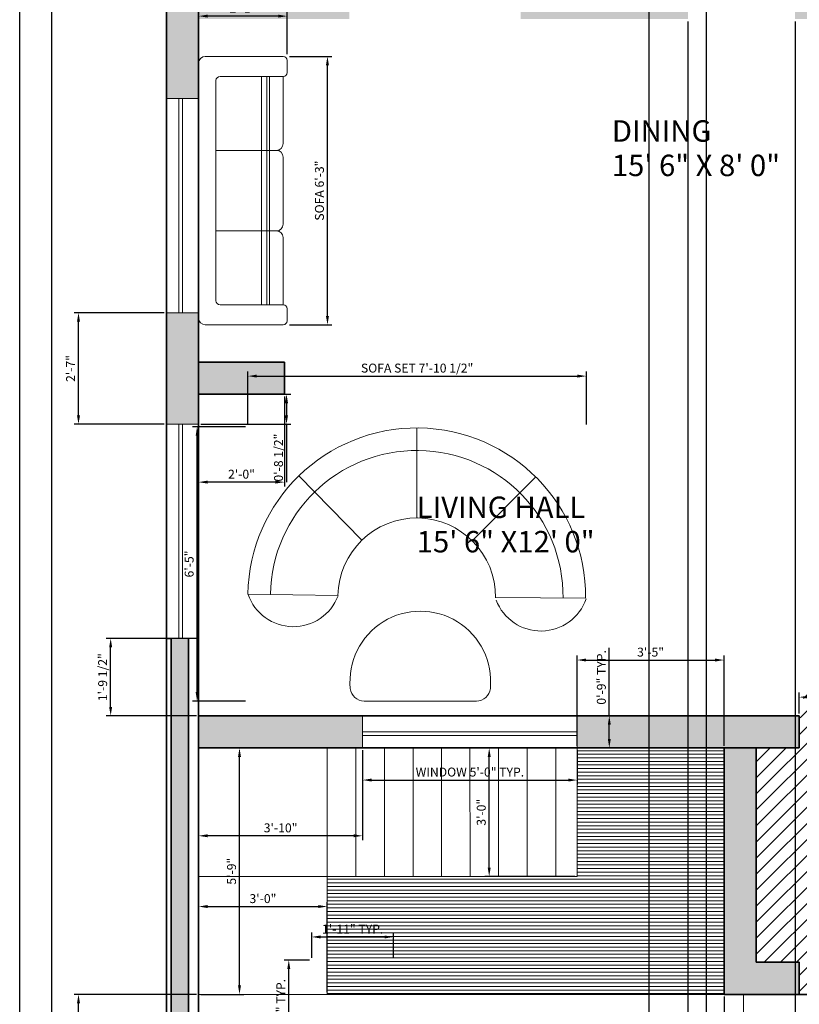
# Model space of a CAD drawing. Units: inches. Extents: x 2998 to 3448, y 1620 to 2377.
# Tile 2 of 5: x 2998 to 3216, y 1879 to 2155. Entities that reach past the tile are written whole.
import ezdxf

# ---------------------------------------------------------------- set-up
doc = ezdxf.new("R2010")
doc.units = ezdxf.units.IN
doc.layers.get('Defpoints').update_dxf_attribs({"color": 110})
for name, color, linetype, lineweight in [('A-ANNO-DIMS', 2, 'Continuous', 18), ('A-ANNO-TTLB', 7, 'Continuous', 25), ('A-AREA-IDEN', 130, 'Continuous', 18), ('A-FLOR-PATT', 18, 'Continuous', 13), ('A-FLOR-STRS', 7, 'Continuous', 18), ('A-GLAZ', 4, 'Continuous', 18), ('A-WALL-PATT', 18, 'Continuous', 13), ('C-PROP', 7, 'Continuous', 35), ('FURNITURE', 8, 'Continuous', 18), ('L-HRDS', 8, 'Continuous', 18), ('L-HRDS-PATT', 175, 'Continuous', 13), ('WALL', 7, 'Continuous', 35)]:
    doc.layers.add(name, color=color, linetype=linetype, lineweight=lineweight)
doc.styles.get("Standard").update_dxf_attribs({"font": 'arial.ttf'})
doc.dimstyles.new('Copy of ISO-25', dxfattribs={"dimtxt": 2.5, "dimasz": 2.5, "dimexe": 1.25, "dimexo": 0.625, "dimtad": 1, "dimdec": 1, "dimlunit": 4, "dimtxsty": 'Standard', "dimcen": 2.5, "dimadec": 0, "dimazin": 0, "dimtfac": 1, "dimtdec": 1, "dimtmove": 0, "dimatfit": 3, "dimfxl": 1, "dimarcsym": 0})

# ---------------------------------------------------------------- blocks, each defined once
blk = doc.blocks.new('*D5')
at = {"layer": 'A-ANNO-DIMS', "color": 0, "lineweight": -2, "transparency": 16777216}
for p, q in [((3048.74, 1950.77), (3060.81, 1950.77)), ((3059.56, 1884.27), (3059.56, 1948.27)), ((3048.74, 1881.77), (3060.81, 1881.77))]:
    blk.add_line(p, q, dxfattribs=at)
at = {"layer": 'A-ANNO-DIMS', "color": 0, "transparency": 16777216}
for points in [[(3059.15, 1948.27), (3059.98, 1948.27), (3059.56, 1950.77)], [(3059.15, 1884.27), (3059.98, 1884.27), (3059.56, 1881.77)]]:
    blk.add_solid(points, dxfattribs=at)
at = {"layer": 'Defpoints', "color": 0, "transparency": 16777216}
for p in [(3048.12, 1950.77), (3059.56, 1950.77), (3048.12, 1881.77)]:
    blk.add_point(p, dxfattribs=at)
at = {"layer": 'A-ANNO-DIMS', "color": 0, "transparency": 16777216, "insert": (3057.66, 1916.27), "char_height": 2.5, "attachment_point": 5, "rotation": 90}
blk.add_mtext('5\'-9"', dxfattribs=at)
blk = doc.blocks.new('A$C22FC404C')
for p, q in [((1199.9, 1301.9), (1199.9, 1941.9)), ((809.2, 1143.1), (362.7, 1601.6)), ((1594.3, 1139.4), (2045.1, 1593.7)), ((0, 760.4), (639.9, 750.6)), ((2399.8, 731.4), (1759.8, 735.4)), ((827.3, 0), (1623.4, 0))]:
    blk.add_line(p, q)
for centre, radius, start, end in [((1199.9, 741.9), 1200, 359.49903, 179.11736), ((1199.9, 741.9), 1040, 359.40957, 179.11736), ((1199.9, 741.9), 560, 359.32862, 179.11736), ((323.1, 869.6), 340.6, 199.13086, 339.10386), ((2082.3, 838.8), 340.6, 200.89614, 340.86914), ((1225.3, 139.3), 500, 354.35827, 185.64173), ((827.3, 100), 100, 185.64173, 270), ((1623.4, 100), 100, 270, 354.35827)]:
    blk.add_arc(centre, radius, start, end)
blk = doc.blocks.new('A$C05BA3A2B')
for p, q in [((0, 0.03), (0, 0.6096)), ((0, 0.03), (0, 0.6096)), ((0, 0.03), (0, 0.6096)), ((0.05, 0.6596), (1.95, 0.6596)), ((0.05, 0.6596), (1.95, 0.6596)), ((0.05, 0.6596), (1.95, 0.6596)), ((2, 0.6096), (2, 0.03)), ((2, 0.6096), (2, 0.03)), ((2, 0.6096), (2, 0.03)), ((1.82, 0.53), (0.18, 0.53)), ((1.82, 0.53), (0.18, 0.53)), ((1.82, 0.53), (0.18, 0.53)), ((0.7, 0.08), (0.7, 0.53)), ((0.7, 0.08), (0.7, 0.53)), ((0.7, 0.08), (0.7, 0.53)), ((1.3, 0.53), (1.3, 0.08)), ((1.3, 0.53), (1.3, 0.08)), ((1.3, 0.53), (1.3, 0.08)), ((0.15, 0.5), (0.15, 0.03)), ((0.15, 0.5), (0.15, 0.03)), ((0.15, 0.5), (0.15, 0.03)), ((1.85, 0.03), (1.85, 0.5)), ((1.85, 0.03), (1.85, 0.5)), ((1.85, 0.03), (1.85, 0.5)), ((1.85, 0.1908), (0.15, 0.1908)), ((1.85, 0.1908), (0.15, 0.1908)), ((1.85, 0.1908), (0.15, 0.1908)), ((1.85, 0.1508), (0.15, 0.1508)), ((1.85, 0.1508), (0.15, 0.1508)), ((1.85, 0.1508), (0.15, 0.1508)), ((1.85, 0.1308), (0.15, 0.1308)), ((1.85, 0.1308), (0.15, 0.1308)), ((1.85, 0.1308), (0.15, 0.1308)), ((0.12, 0), (0.03, 0)), ((0.12, 0), (0.03, 0)), ((0.12, 0), (0.03, 0)), ((0.65, 0.03), (0.15, 0.03)), ((0.65, 0.03), (0.15, 0.03)), ((0.65, 0.03), (0.15, 0.03)), ((1.25, 0.03), (0.75, 0.03)), ((1.25, 0.03), (0.75, 0.03)), ((1.25, 0.03), (0.75, 0.03)), ((1.85, 0.03), (1.35, 0.03)), ((1.85, 0.03), (1.35, 0.03)), ((1.85, 0.03), (1.35, 0.03)), ((1.97, 0), (1.88, 0)), ((1.97, 0), (1.88, 0)), ((1.97, 0), (1.88, 0))]:
    blk.add_line(p, q)
for centre, radius, start, end in [((0.05, 0.6096), 0.05, 90, 180), ((0.05, 0.6096), 0.05, 90, 180), ((0.05, 0.6096), 0.05, 90, 180), ((1.95, 0.6096), 0.05, 0, 90), ((1.95, 0.6096), 0.05, 0, 90), ((1.95, 0.6096), 0.05, 0, 90), ((0.18, 0.5), 0.03, 90, 180), ((0.18, 0.5), 0.03, 90, 180), ((0.18, 0.5), 0.03, 90, 180), ((1.82, 0.5), 0.03, 0, 90), ((1.82, 0.5), 0.03, 0, 90), ((1.82, 0.5), 0.03, 0, 90), ((0.65, 0.08), 0.05, 270, 0), ((0.65, 0.08), 0.05, 270, 0), ((0.65, 0.08), 0.05, 270, 0), ((0.75, 0.08), 0.05, 180, 270), ((0.75, 0.08), 0.05, 180, 270), ((0.75, 0.08), 0.05, 180, 270), ((1.25, 0.08), 0.05, 270, 0), ((1.25, 0.08), 0.05, 270, 0), ((1.25, 0.08), 0.05, 270, 0), ((1.35, 0.08), 0.05, 180, 270), ((1.35, 0.08), 0.05, 180, 270), ((1.35, 0.08), 0.05, 180, 270), ((0.03, 0.03), 0.03, 180, 270), ((0.03, 0.03), 0.03, 180, 270), ((0.03, 0.03), 0.03, 180, 270), ((0.12, 0.03), 0.03, 270, 0), ((0.12, 0.03), 0.03, 270, 0), ((0.12, 0.03), 0.03, 270, 0), ((1.88, 0.03), 0.03, 180, 270), ((1.88, 0.03), 0.03, 180, 270), ((1.88, 0.03), 0.03, 180, 270), ((1.97, 0.03), 0.03, 270, 0), ((1.97, 0.03), 0.03, 270, 0), ((1.97, 0.03), 0.03, 270, 0)]:
    blk.add_arc(centre, radius, start, end)
blk = doc.blocks.new('*D20')
at = {"layer": 'A-ANNO-DIMS', "color": 0, "lineweight": -2, "transparency": 16777216}
for p, q in [((3216.12, 1960.4), (3216.12, 1966.24)), ((3252.12, 1960.4), (3252.12, 1966.24)), ((3218.62, 1964.99), (3249.62, 1964.99))]:
    blk.add_line(p, q, dxfattribs=at)
at = {"layer": 'A-ANNO-DIMS', "color": 0, "transparency": 16777216}
for points in [[(3218.62, 1965.4), (3218.62, 1964.57), (3216.12, 1964.99)], [(3249.62, 1965.4), (3249.62, 1964.57), (3252.12, 1964.99)]]:
    blk.add_solid(points, dxfattribs=at)
at = {"layer": 'Defpoints', "color": 0, "transparency": 16777216}
for p in [(3252.12, 1964.99), (3216.12, 1959.77), (3252.12, 1959.77)]:
    blk.add_point(p, dxfattribs=at)
at = {"layer": 'A-ANNO-DIMS', "color": 0, "transparency": 16777216, "insert": (3234.12, 1966.89), "char_height": 2.5, "attachment_point": 5}
blk.add_mtext("3'", dxfattribs=at)
blk = doc.blocks.new('WIN-60IN')
for p, q in [((0, 0), (0, 9)), ((60, 9), (60, 0)), ((0, 4.5), (60, 4.5)), ((0, 3.5), (60, 3.5))]:
    blk.add_line(p, q)
blk = doc.blocks.new('*D27')
at = {"layer": 'A-ANNO-DIMS', "color": 0, "lineweight": -2, "transparency": 16777216}
for p, q in [((3079.17, 1891.4), (3072.1, 1891.4)), ((3073.35, 1850.88), (3073.35, 1888.9)), ((3079.17, 1848.38), (3072.1, 1848.38))]:
    blk.add_line(p, q, dxfattribs=at)
at = {"layer": 'A-ANNO-DIMS', "color": 0, "transparency": 16777216}
for points in [[(3072.93, 1888.9), (3073.76, 1888.9), (3073.35, 1891.4)], [(3072.93, 1850.88), (3073.76, 1850.88), (3073.35, 1848.38)]]:
    blk.add_solid(points, dxfattribs=at)
at = {"layer": 'Defpoints', "color": 0}
for p in [(3073.35, 1891.4), (3079.8, 1891.4), (3079.8, 1848.38)]:
    blk.add_point(p, dxfattribs=at)
at = {"layer": 'A-ANNO-DIMS', "color": 0, "transparency": 16777216, "insert": (3071.43, 1869.89), "char_height": 2.5, "attachment_point": 5, "rotation": 90}
blk.add_mtext('PLANTING 3\'-7" TYP.', dxfattribs=at)
blk = doc.blocks.new('*D28')
at = {"layer": 'A-ANNO-DIMS', "color": 0, "lineweight": -2, "transparency": 16777216}
for p, q in [((3079.8, 1892.03), (3079.8, 1899.11)), ((3102.63, 1892.03), (3102.63, 1899.11)), ((3082.3, 1897.86), (3100.13, 1897.86))]:
    blk.add_line(p, q, dxfattribs=at)
at = {"layer": 'A-ANNO-DIMS', "color": 0, "transparency": 16777216}
for points in [[(3082.3, 1898.28), (3082.3, 1897.44), (3079.8, 1897.86)], [(3100.13, 1898.28), (3100.13, 1897.44), (3102.63, 1897.86)]]:
    blk.add_solid(points, dxfattribs=at)
at = {"layer": 'Defpoints', "color": 0}
for p in [(3102.63, 1897.86), (3079.8, 1891.4), (3102.63, 1891.4)]:
    blk.add_point(p, dxfattribs=at)
at = {"layer": 'A-ANNO-DIMS', "color": 0, "transparency": 16777216, "insert": (3091.22, 1899.74), "char_height": 2.5, "attachment_point": 5}
blk.add_mtext('1\'-11" TYP.', dxfattribs=at)
blk = doc.blocks.new('*D29')
at = {"layer": 'A-ANNO-DIMS', "color": 0, "lineweight": -2, "transparency": 16777216}
for p, q in [((3094.02, 1950.15), (3094.02, 1940.52)), ((3154.02, 1950.15), (3154.02, 1940.52)), ((3096.52, 1941.77), (3151.52, 1941.77))]:
    blk.add_line(p, q, dxfattribs=at)
at = {"layer": 'A-ANNO-DIMS', "color": 0, "transparency": 16777216}
for points in [[(3096.52, 1942.19), (3096.52, 1941.36), (3094.02, 1941.77)], [(3151.52, 1942.19), (3151.52, 1941.36), (3154.02, 1941.77)]]:
    blk.add_solid(points, dxfattribs=at)
at = {"layer": 'Defpoints', "color": 0}
for p in [(3094.02, 1950.77), (3154.02, 1950.77), (3154.02, 1941.77)]:
    blk.add_point(p, dxfattribs=at)
at = {"layer": 'A-ANNO-DIMS', "color": 0, "transparency": 16777216, "insert": (3124.02, 1943.69), "char_height": 2.5, "attachment_point": 5}
blk.add_mtext('WINDOW 5\'-0" TYP.', dxfattribs=at)
blk = doc.blocks.new('*D30')
at = {"layer": 'A-ANNO-DIMS', "color": 0, "lineweight": -2, "transparency": 16777216}
for p, q in [((3163.02, 1959.77), (3163.02, 1978.76)), ((3154.65, 1959.77), (3164.27, 1959.77)), ((3163.02, 1953.27), (3163.02, 1957.27)), ((3154.65, 1950.77), (3164.27, 1950.77))]:
    blk.add_line(p, q, dxfattribs=at)
at = {"layer": 'A-ANNO-DIMS', "color": 0, "transparency": 16777216}
for points in [[(3162.61, 1957.27), (3163.44, 1957.27), (3163.02, 1959.77)], [(3162.61, 1953.27), (3163.44, 1953.27), (3163.02, 1950.77)]]:
    blk.add_solid(points, dxfattribs=at)
at = {"layer": 'Defpoints', "color": 0}
for p in [(3154.02, 1959.77), (3163.02, 1959.77), (3154.02, 1950.77)]:
    blk.add_point(p, dxfattribs=at)
at = {"layer": 'A-ANNO-DIMS', "color": 0, "transparency": 16777216, "insert": (3161.12, 1970.52), "char_height": 2.5, "attachment_point": 5, "rotation": 90}
blk.add_mtext('0\'-9" TYP.', dxfattribs=at)
blk = doc.blocks.new('*D35')
at = {"layer": 'A-ANNO-DIMS', "color": 0, "lineweight": -2, "transparency": 16777216}
for p, q in [((3061.91, 2041.27), (3061.91, 2056.1)), ((3156.62, 2041.27), (3156.62, 2056.1)), ((3064.41, 2054.85), (3154.12, 2054.85))]:
    blk.add_line(p, q, dxfattribs=at)
at = {"layer": 'A-ANNO-DIMS', "color": 0, "transparency": 16777216}
for points in [[(3064.41, 2055.27), (3064.41, 2054.43), (3061.91, 2054.85)], [(3154.12, 2055.27), (3154.12, 2054.43), (3156.62, 2054.85)]]:
    blk.add_solid(points, dxfattribs=at)
at = {"layer": 'Defpoints', "color": 0}
for p in [(3156.62, 2054.85), (3061.91, 2040.64), (3156.62, 2040.64)]:
    blk.add_point(p, dxfattribs=at)
at = {"layer": 'A-ANNO-DIMS', "color": 0, "transparency": 16777216, "insert": (3109.26, 2056.77), "char_height": 2.5, "attachment_point": 5}
blk.add_mtext('SOFA SET 7\'-10 1/2"', dxfattribs=at)
blk = doc.blocks.new('*D36')
at = {"layer": 'A-ANNO-DIMS', "color": 0, "lineweight": -2, "transparency": 16777216}
for p, q in [((3061.28, 2040.64), (3046.45, 2040.64)), ((3047.7, 1966.38), (3047.7, 2038.14)), ((3061.28, 1963.88), (3046.45, 1963.88))]:
    blk.add_line(p, q, dxfattribs=at)
at = {"layer": 'A-ANNO-DIMS', "color": 0, "transparency": 16777216}
for points in [[(3047.29, 2038.14), (3048.12, 2038.14), (3047.7, 2040.64)], [(3047.29, 1966.38), (3048.12, 1966.38), (3047.7, 1963.88)]]:
    blk.add_solid(points, dxfattribs=at)
at = {"layer": 'Defpoints', "color": 0}
for p in [(3047.7, 2040.64), (3061.91, 2040.64), (3061.91, 1963.88)]:
    blk.add_point(p, dxfattribs=at)
at = {"layer": 'A-ANNO-DIMS', "color": 0, "transparency": 16777216, "insert": (3045.8, 2002.26), "char_height": 2.5, "attachment_point": 5, "rotation": 90}
blk.add_mtext('6\'-5"', dxfattribs=at)
blk = doc.blocks.new('*D37')
at = {"layer": 'A-ANNO-DIMS', "color": 0, "lineweight": -2, "transparency": 16777216}
for p, q in [((3073.53, 2144.34), (3085.42, 2144.34)), ((3084.17, 2071.7), (3084.17, 2141.84)), ((3073.53, 2069.2), (3085.42, 2069.2))]:
    blk.add_line(p, q, dxfattribs=at)
at = {"layer": 'A-ANNO-DIMS', "color": 0, "transparency": 16777216}
for points in [[(3083.75, 2141.84), (3084.59, 2141.84), (3084.17, 2144.34)], [(3083.75, 2071.7), (3084.59, 2071.7), (3084.17, 2069.2)]]:
    blk.add_solid(points, dxfattribs=at)
at = {"layer": 'Defpoints', "color": 0}
for p in [(3072.9, 2144.34), (3084.17, 2144.34), (3072.9, 2069.2)]:
    blk.add_point(p, dxfattribs=at)
at = {"layer": 'A-ANNO-DIMS', "color": 0, "transparency": 16777216, "insert": (3082.25, 2106.77), "char_height": 2.5, "attachment_point": 5, "rotation": 90}
blk.add_mtext('SOFA 6\'-3"', dxfattribs=at)
blk = doc.blocks.new('*D38')
at = {"layer": 'A-ANNO-DIMS', "color": 0, "lineweight": -2, "transparency": 16777216}
for p, q in [((3048.12, 2144.97), (3048.12, 2156.87)), ((3070.4, 2155.62), (3050.62, 2155.62)), ((3072.9, 2144.97), (3072.9, 2156.87))]:
    blk.add_line(p, q, dxfattribs=at)
at = {"layer": 'A-ANNO-DIMS', "color": 0, "transparency": 16777216}
for points in [[(3050.62, 2156.03), (3050.62, 2155.2), (3048.12, 2155.62)], [(3070.4, 2156.03), (3070.4, 2155.2), (3072.9, 2155.62)]]:
    blk.add_solid(points, dxfattribs=at)
at = {"layer": 'Defpoints', "color": 0}
for p in [(3048.12, 2155.62), (3048.12, 2144.34), (3072.9, 2144.34)]:
    blk.add_point(p, dxfattribs=at)
at = {"layer": 'A-ANNO-DIMS', "color": 0, "transparency": 16777216, "insert": (3060.51, 2157.5), "char_height": 2.5, "attachment_point": 5}
blk.add_mtext('2\'-1"', dxfattribs=at)
blk = doc.blocks.new('*D42')
at = {"layer": 'A-ANNO-DIMS', "color": 0, "lineweight": -2, "transparency": 16777216}
for p, q in [((3047.49, 1881.77), (3013.27, 1881.77)), ((3014.52, 1854.27), (3014.52, 1879.27)), ((3047.49, 1851.77), (3013.27, 1851.77))]:
    blk.add_line(p, q, dxfattribs=at)
at = {"layer": 'A-ANNO-DIMS', "color": 0, "transparency": 16777216}
for points in [[(3014.1, 1879.27), (3014.94, 1879.27), (3014.52, 1881.77)], [(3014.1, 1854.27), (3014.94, 1854.27), (3014.52, 1851.77)]]:
    blk.add_solid(points, dxfattribs=at)
at = {"layer": 'Defpoints', "color": 0}
for p in [(3014.52, 1881.77), (3048.12, 1881.77), (3048.12, 1851.77)]:
    blk.add_point(p, dxfattribs=at)
at = {"layer": 'A-ANNO-DIMS', "color": 0, "transparency": 16777216, "insert": (3012.62, 1866.77), "char_height": 2.5, "attachment_point": 5, "rotation": 90}
blk.add_mtext('2\'-6"', dxfattribs=at)
blk = doc.blocks.new('*D43')
at = {"layer": 'A-ANNO-DIMS', "color": 0, "lineweight": -2, "transparency": 16777216}
for p, q in [((3048.12, 1881.15), (3048.12, 1816.92)), ((3195.12, 1881.15), (3195.12, 1816.92)), ((3050.62, 1818.17), (3192.62, 1818.17))]:
    blk.add_line(p, q, dxfattribs=at)
at = {"layer": 'A-ANNO-DIMS', "color": 0, "transparency": 16777216}
for points in [[(3050.62, 1818.59), (3050.62, 1817.76), (3048.12, 1818.17)], [(3192.62, 1818.59), (3192.62, 1817.76), (3195.12, 1818.17)]]:
    blk.add_solid(points, dxfattribs=at)
at = {"layer": 'Defpoints', "color": 0}
for p in [(3048.12, 1881.77), (3195.12, 1881.77), (3195.12, 1818.17)]:
    blk.add_point(p, dxfattribs=at)
at = {"layer": 'A-ANNO-DIMS', "color": 0, "transparency": 16777216, "insert": (3121.62, 1820.07), "char_height": 2.5, "attachment_point": 5}
blk.add_mtext('12\'-3"', dxfattribs=at)
blk = doc.blocks.new('*D51')
at = {"layer": 'A-ANNO-DIMS', "color": 0, "lineweight": -2, "transparency": 16777216}
for p, q in [((3174.12, 2256.15), (3174.12, 1816.92)), ((3190.13, 2256.15), (3190.13, 1816.92)), ((3176.62, 1818.17), (3187.63, 1818.17))]:
    blk.add_line(p, q, dxfattribs=at)
at = {"layer": 'A-ANNO-DIMS', "color": 0, "transparency": 16777216}
for points in [[(3176.62, 1818.59), (3176.62, 1817.76), (3174.12, 1818.17)], [(3187.63, 1818.59), (3187.63, 1817.76), (3190.13, 1818.17)]]:
    blk.add_solid(points, dxfattribs=at)
at = {"layer": 'Defpoints', "color": 0}
for p in [(3174.12, 2256.77), (3190.13, 2256.77), (3190.13, 1818.17)]:
    blk.add_point(p, dxfattribs=at)
at = {"layer": 'A-ANNO-DIMS', "color": 0, "transparency": 16777216, "insert": (3182.12, 1820.05), "char_height": 2.5, "attachment_point": 5}
blk.add_mtext('1\'-4"', dxfattribs=at)
blk = doc.blocks.new('*D54')
at = {"layer": 'A-ANNO-DIMS', "color": 0, "lineweight": -2, "transparency": 16777216}
for p, q in [((3185.01, 2154.15), (3185.01, 1816.92)), ((3215.01, 2154.15), (3215.01, 1816.92)), ((3187.51, 1818.17), (3212.51, 1818.17))]:
    blk.add_line(p, q, dxfattribs=at)
at = {"layer": 'A-ANNO-DIMS', "color": 0, "transparency": 16777216}
for points in [[(3187.51, 1818.59), (3187.51, 1817.76), (3185.01, 1818.17)], [(3212.51, 1818.59), (3212.51, 1817.76), (3215.01, 1818.17)]]:
    blk.add_solid(points, dxfattribs=at)
at = {"layer": 'Defpoints', "color": 0}
for p in [(3185.01, 2154.77), (3215.01, 2154.77), (3215.01, 1818.17)]:
    blk.add_point(p, dxfattribs=at)
at = {"layer": 'A-ANNO-DIMS', "color": 0, "transparency": 16777216, "insert": (3200.01, 1820.07), "char_height": 2.5, "attachment_point": 5}
blk.add_mtext('2\'-6"', dxfattribs=at)
blk = doc.blocks.new('*D63')
at = {"layer": 'A-ANNO-DIMS', "color": 0, "lineweight": -2, "transparency": 16777216}
for p, q in [((3038.49, 2072.57), (3013.27, 2072.57)), ((3014.52, 2043.9), (3014.52, 2070.07)), ((3038.49, 2041.4), (3013.27, 2041.4))]:
    blk.add_line(p, q, dxfattribs=at)
at = {"layer": 'A-ANNO-DIMS', "color": 0, "transparency": 16777216}
for points in [[(3014.1, 2070.07), (3014.94, 2070.07), (3014.52, 2072.57)], [(3014.1, 2043.9), (3014.94, 2043.9), (3014.52, 2041.4)]]:
    blk.add_solid(points, dxfattribs=at)
at = {"layer": 'Defpoints', "color": 0}
for p in [(3014.52, 2072.57), (3039.12, 2072.57), (3039.12, 2041.4)]:
    blk.add_point(p, dxfattribs=at)
at = {"layer": 'A-ANNO-DIMS', "color": 0, "transparency": 16777216, "insert": (3012.64, 2056.98), "char_height": 2.5, "attachment_point": 5, "rotation": 90}
blk.add_mtext('2\'-7"', dxfattribs=at)
blk = doc.blocks.new('*D64')
at = {"layer": 'A-ANNO-DIMS', "color": 0, "lineweight": -2, "transparency": 16777216}
for p, q in [((3047.49, 1981.4), (3022.27, 1981.4)), ((3023.52, 1962.27), (3023.52, 1978.9)), ((3047.49, 1959.77), (3022.27, 1959.77))]:
    blk.add_line(p, q, dxfattribs=at)
at = {"layer": 'A-ANNO-DIMS', "color": 0, "transparency": 16777216}
for points in [[(3023.1, 1978.9), (3023.94, 1978.9), (3023.52, 1981.4)], [(3023.1, 1962.27), (3023.94, 1962.27), (3023.52, 1959.77)]]:
    blk.add_solid(points, dxfattribs=at)
at = {"layer": 'Defpoints', "color": 0}
for p in [(3023.52, 1981.4), (3048.12, 1981.4), (3048.12, 1959.77)]:
    blk.add_point(p, dxfattribs=at)
at = {"layer": 'A-ANNO-DIMS', "color": 0, "transparency": 16777216, "insert": (3021.6, 1970.58), "char_height": 2.5, "attachment_point": 5, "rotation": 90}
blk.add_mtext('1\'-9 1/2"', dxfattribs=at)
blk = doc.blocks.new('*D65')
at = {"layer": 'A-ANNO-DIMS', "color": 0, "lineweight": -2, "transparency": 16777216}
for p, q in [((3048.12, 1950.15), (3048.12, 1924.92)), ((3094.02, 1950.15), (3094.02, 1924.92)), ((3091.52, 1926.17), (3050.62, 1926.17))]:
    blk.add_line(p, q, dxfattribs=at)
at = {"layer": 'A-ANNO-DIMS', "color": 0, "transparency": 16777216}
for points in [[(3050.62, 1926.59), (3050.62, 1925.76), (3048.12, 1926.17)], [(3091.52, 1926.59), (3091.52, 1925.76), (3094.02, 1926.17)]]:
    blk.add_solid(points, dxfattribs=at)
at = {"layer": 'Defpoints', "color": 0}
for p in [(3048.12, 1950.77), (3094.02, 1950.77), (3048.12, 1926.17)]:
    blk.add_point(p, dxfattribs=at)
at = {"layer": 'A-ANNO-DIMS', "color": 0, "transparency": 16777216, "insert": (3071.07, 1928.07), "char_height": 2.5, "attachment_point": 5}
blk.add_mtext('3\'-10"', dxfattribs=at)
blk = doc.blocks.new('*D70')
at = {"layer": 'A-ANNO-DIMS', "color": 0, "lineweight": -2, "transparency": 16777216}
for p, q in [((3048.12, 1882.4), (3048.12, 1907.62)), ((3084.12, 1882.4), (3084.12, 1907.62)), ((3050.62, 1906.37), (3081.62, 1906.37))]:
    blk.add_line(p, q, dxfattribs=at)
at = {"layer": 'A-ANNO-DIMS', "color": 0, "transparency": 16777216}
for points in [[(3050.62, 1906.79), (3050.62, 1905.96), (3048.12, 1906.37)], [(3081.62, 1906.79), (3081.62, 1905.96), (3084.12, 1906.37)]]:
    blk.add_solid(points, dxfattribs=at)
at = {"layer": 'Defpoints', "color": 0}
for p in [(3084.12, 1906.37), (3048.12, 1881.77), (3084.12, 1881.77)]:
    blk.add_point(p, dxfattribs=at)
at = {"layer": 'A-ANNO-DIMS', "color": 0, "transparency": 16777216, "insert": (3066.12, 1908.27), "char_height": 2.5, "attachment_point": 5}
blk.add_mtext('3\'-0"', dxfattribs=at)
blk = doc.blocks.new('*D71')
at = {"layer": 'A-ANNO-DIMS', "color": 0, "lineweight": -2, "transparency": 16777216}
for p, q in [((3153.4, 1950.77), (3128.17, 1950.77)), ((3129.42, 1917.27), (3129.42, 1948.27)), ((3153.4, 1914.77), (3128.17, 1914.77))]:
    blk.add_line(p, q, dxfattribs=at)
at = {"layer": 'A-ANNO-DIMS', "color": 0, "transparency": 16777216}
for points in [[(3129.01, 1948.27), (3129.84, 1948.27), (3129.42, 1950.77)], [(3129.01, 1917.27), (3129.84, 1917.27), (3129.42, 1914.77)]]:
    blk.add_solid(points, dxfattribs=at)
at = {"layer": 'Defpoints', "color": 0}
for p in [(3129.42, 1950.77), (3154.02, 1950.77), (3154.02, 1914.77)]:
    blk.add_point(p, dxfattribs=at)
at = {"layer": 'A-ANNO-DIMS', "color": 0, "transparency": 16777216, "insert": (3127.52, 1932.77), "char_height": 2.5, "attachment_point": 5, "rotation": 90}
blk.add_mtext('3\'-0"', dxfattribs=at)
blk = doc.blocks.new('*D72')
at = {"layer": 'A-ANNO-DIMS', "color": 0, "lineweight": -2, "transparency": 16777216}
for p, q in [((3154.02, 1951.4), (3154.02, 1976.62)), ((3195.12, 1951.4), (3195.12, 1976.62)), ((3156.52, 1975.37), (3192.62, 1975.37))]:
    blk.add_line(p, q, dxfattribs=at)
at = {"layer": 'A-ANNO-DIMS', "color": 0, "transparency": 16777216}
for points in [[(3156.52, 1975.79), (3156.52, 1974.96), (3154.02, 1975.37)], [(3192.62, 1975.79), (3192.62, 1974.96), (3195.12, 1975.37)]]:
    blk.add_solid(points, dxfattribs=at)
at = {"layer": 'Defpoints', "color": 0}
for p in [(3195.12, 1975.37), (3154.02, 1950.77), (3195.12, 1950.77)]:
    blk.add_point(p, dxfattribs=at)
at = {"layer": 'A-ANNO-DIMS', "color": 0, "transparency": 16777216, "insert": (3174.57, 1977.27), "char_height": 2.5, "attachment_point": 5}
blk.add_mtext('3\'-5"', dxfattribs=at)
blk = doc.blocks.new('*D74')
at = {"layer": 'A-ANNO-DIMS', "color": 0, "lineweight": -2, "transparency": 16777216}
for p, q in [((3048.74, 2049.77), (3073.97, 2049.77)), ((3072.72, 2047.27), (3072.72, 2043.9)), ((3048.74, 2041.4), (3073.97, 2041.4)), ((3072.72, 2041.4), (3072.72, 2025.18))]:
    blk.add_line(p, q, dxfattribs=at)
at = {"layer": 'A-ANNO-DIMS', "color": 0, "transparency": 16777216}
for points in [[(3072.3, 2047.27), (3073.14, 2047.27), (3072.72, 2049.77)], [(3072.3, 2043.9), (3073.14, 2043.9), (3072.72, 2041.4)]]:
    blk.add_solid(points, dxfattribs=at)
at = {"layer": 'Defpoints', "color": 0}
for p in [(3048.12, 2049.77), (3048.12, 2041.4), (3072.72, 2041.4)]:
    blk.add_point(p, dxfattribs=at)
at = {"layer": 'A-ANNO-DIMS', "color": 0, "transparency": 16777216, "insert": (3070.8, 2032.04), "char_height": 2.5, "attachment_point": 5, "rotation": 90}
blk.add_mtext('0\'-8 1/2"', dxfattribs=at)
blk = doc.blocks.new('*D75')
at = {"layer": 'A-ANNO-DIMS', "color": 0, "lineweight": -2, "transparency": 16777216}
for p, q in [((3048.12, 2049.15), (3048.12, 2023.92)), ((3072.12, 2049.15), (3072.12, 2023.92)), ((3069.62, 2025.17), (3050.62, 2025.17))]:
    blk.add_line(p, q, dxfattribs=at)
at = {"layer": 'A-ANNO-DIMS', "color": 0, "transparency": 16777216}
for points in [[(3050.62, 2025.59), (3050.62, 2024.76), (3048.12, 2025.17)], [(3069.62, 2025.59), (3069.62, 2024.76), (3072.12, 2025.17)]]:
    blk.add_solid(points, dxfattribs=at)
at = {"layer": 'Defpoints', "color": 0}
for p in [(3048.12, 2049.77), (3072.12, 2049.77), (3048.12, 2025.17)]:
    blk.add_point(p, dxfattribs=at)
at = {"layer": 'A-ANNO-DIMS', "color": 0, "transparency": 16777216, "insert": (3060.12, 2027.07), "char_height": 2.5, "attachment_point": 5}
blk.add_mtext('2\'-0"', dxfattribs=at)

msp = doc.modelspace()

# ---------------------------------------------------------------- hatches: boundary and pattern name
at = {"layer": 'A-FLOR-PATT'}
h = msp.add_hatch(dxfattribs=at)
h.set_pattern_fill('ANSI31', color=256)
h.paths.add_polyline_path([(3264.12, 1950.77), (3252.12, 1950.77), (3252.12, 1955.56), (3250.03, 1955.56), (3250.03, 1991.39, 0.39722), (3216.23, 1955.56), (3216.23, 1950.77), (3204.12, 1950.77), (3204.12, 1890.77), (3216.12, 1890.77), (3216.12, 1881.77), (3252.12, 1881.77), (3252.12, 1890.77), (3264.12, 1890.77)])
h.paths.add_polyline_path([(3343.37, 2313.77), (3048.12, 2313.77), (3048.12, 2265.77), (3059.91, 2265.77), (3059.91, 2296.51), (3061.95, 2296.51), (3061.95, 2296.45, -0.39722), (3094.97, 2261.45), (3095.91, 2265.77), (3343.37, 2265.77)])
h.paths.add_polyline_path([(3220.44, 1918.61), (3261.55, 1918.61), (3261.55, 1927.8), (3220.44, 1927.8)], flags=24)
h.paths.add_polyline_path([(3220.42, 1928.23), (3252.4, 1928.23), (3252.4, 1937.54), (3220.42, 1937.54)], flags=24)
h.paths.add_polyline_path([(3097.58, 2294.93), (3164.02, 2294.93), (3164.02, 2304.23), (3097.58, 2304.23)], flags=24)
at = {"layer": 'A-WALL-PATT'}
h = msp.add_hatch(color=256, dxfattribs=at)
h.dxf.hatch_style = 1
h.paths.add_polyline_path([(3399.12, 2322.77), (3039.12, 2322.77), (3039.12, 2132.57), (3048.12, 2132.57), (3048.12, 2154.77), (3048.12, 2313.77), (3390.12, 2313.77), (3390.12, 2227.86), (3399.12, 2227.86)])
h.paths.add_polyline_path([(3048.12, 2072.57), (3039.12, 2072.57), (3039.12, 2041.4), (3048.12, 2041.4)])
h.paths.add_polyline_path([(3399.12, 1997.2), (3390.12, 1997.2), (3390.12, 1851.77), (3274.41, 1851.77), (3274.41, 1842.77), (3399.12, 1842.77)])
h.paths.add_polyline_path([(3195.35, 1851.77), (3048.12, 1851.77), (3048.12, 1857.27), (3048.05, 1858.06), (3047.68, 1858.02), (3047.44, 1857.61), (3047.47, 1857.28), (3047.17, 1857.15), (3047.68, 1858.02), (3045.29, 1857.73), (3045.29, 1842.77), (3195.35, 1842.77)])
h.paths.add_polyline_path([(3399.12, 2167.86), (3390.12, 2167.86), (3390.12, 2112.77), (3390.12, 2103.77), (3390.12, 2045.2), (3399.12, 2045.2)])
h.paths.add_polyline_path([(3390.12, 2112.77), (3306.12, 2112.77), (3306.12, 2118.77), (3304.88, 2118.77), (3300.12, 2118.77), (3300.12, 2112.77), (3300.12, 2103.77), (3390.12, 2103.77)])
h.paths.add_polyline_path([(3257.48, 2265.77), (3214.13, 2265.77), (3214.13, 2256.77), (3257.48, 2256.77)], flags=17)
h.paths.add_polyline_path([(3325.36, 2265.77), (3281.48, 2265.77), (3281.48, 2256.77), (3300.12, 2256.77), (3325.36, 2256.77)], flags=17)
h.paths.add_polyline_path([(3390.12, 2265.77), (3373.36, 2265.77), (3373.36, 2256.77), (3390.12, 2256.77)], flags=17)
h.paths.add_polyline_path([(3190.13, 2265.77), (3155.91, 2265.77), (3155.91, 2256.77), (3190.13, 2256.77)], flags=17)
h.paths.add_polyline_path([(3306.12, 2256.77), (3300.12, 2256.77), (3300.12, 2160.77), (3298.12, 2160.77), (3298.12, 2154.77), (3300.12, 2154.77), (3306.12, 2154.77)], flags=17)
h.paths.add_polyline_path([(3240.12, 2256.77), (3234.12, 2256.77), (3234.12, 2160.77), (3215.01, 2160.77), (3215.01, 2154.77), (3268.12, 2154.77), (3268.12, 2158.71), (3268.12, 2160.77), (3240.12, 2160.77)], flags=17)
h.paths.add_polyline_path([(3174.12, 2256.77), (3168.12, 2256.77), (3168.12, 2160.77), (3138.26, 2160.77), (3138.26, 2154.77), (3174.12, 2154.77), (3185.01, 2154.77), (3185.01, 2158.71), (3185.01, 2160.77), (3174.12, 2160.77)], flags=17)
h.paths.add_polyline_path([(3090.26, 2160.77), (3048.12, 2160.77), (3048.12, 2154.77), (3090.26, 2154.77)], flags=17)
h.paths.add_polyline_path([(3072.12, 2058.77), (3048.12, 2058.77), (3048.12, 2049.77), (3072.12, 2049.77)])
h.paths.add_polyline_path([(3298.3, 1959.77), (3270.12, 1959.77), (3270.12, 2061.77), (3300.12, 2061.77), (3306.12, 2061.77), (3306.12, 2067.77), (3300.12, 2067.77), (3264.12, 2067.77), (3264.12, 2061.77), (3264.12, 1959.77), (3252.12, 1959.77), (3252.12, 1955.56), (3252.12, 1950.77), (3264.12, 1950.77), (3264.12, 1890.77), (3264.12, 1881.77), (3273.12, 1881.77), (3273.12, 1950.77), (3298.3, 1950.77)])
h.paths.add_polyline_path([(3390.12, 1959.77), (3358.3, 1959.77), (3358.3, 1950.77), (3390.12, 1950.77)], flags=17)
h.paths.add_polyline_path([(3216.12, 1959.77), (3154.02, 1959.77), (3154.02, 1950.77), (3216.12, 1950.77)])
h.paths.add_polyline_path([(3204.12, 1950.77), (3195.12, 1950.77), (3195.12, 1890.77), (3195.12, 1881.77), (3216.12, 1881.77), (3216.12, 1890.77), (3204.12, 1890.77)])
h.paths.add_polyline_path([(3094.02, 1959.77), (3048.12, 1959.77), (3048.12, 1950.77), (3094.02, 1950.77)])
h.paths.add_polyline_path([(3045.29, 1981.4), (3040.45, 1981.4), (3040.45, 1842.77), (3045.29, 1842.77), (3045.29, 1857.73)])
h.paths.add_polyline_path([(3059.91, 2261.45), (3059.91, 2265.77), (3048.12, 2265.77), (3048.12, 2256.77), (3059.91, 2256.77)], flags=17)
h.paths.add_polyline_path([(3107.91, 2265.77), (3095.91, 2265.77), (3095.91, 2256.77), (3107.91, 2256.77)], flags=17)
h.paths.add_polyline_path([(3274.41, 1851.77), (3264.12, 1851.77), (3264.12, 1846.71), (3264.12, 1842.77), (3274.41, 1842.77)])
h.paths.add_polyline_path([(3204.35, 1851.77), (3195.35, 1851.77), (3195.35, 1842.77), (3204.35, 1842.77), (3204.35, 1846.71)])
at = {"layer": 'L-HRDS-PATT'}
h = msp.add_hatch(dxfattribs=at)
h.set_pattern_fill('_USER', color=256, pattern_type=0)
h.set_pattern_definition([(0, (0, 0), (0, 1), [])])
h.paths.add_polyline_path([(3195.12, 1950.77), (3154.02, 1950.77), (3154.02, 1914.77), (3084.12, 1914.77), (3084.12, 1881.77), (3195.12, 1881.77), (3195.12, 1890.77)])
h.paths.add_polyline_path([(3107.62, 2003.86), (3160.38, 2003.86), (3160.38, 2013.05), (3107.62, 2013.05)], flags=9)
h.paths.add_polyline_path([(3107.6, 2013.48), (3161.48, 2013.48), (3161.48, 2022.79), (3107.6, 2022.79)], flags=9)
h.paths.add_polyline_path([(3162.21, 2109.19), (3212.64, 2109.19), (3212.64, 2118.38), (3162.21, 2118.38)], flags=9)
h.paths.add_polyline_path([(3162.19, 2118.81), (3194.63, 2118.81), (3194.63, 2128.12), (3162.19, 2128.12)], flags=9)
h.paths.add_polyline_path([(3334.58, 2144.47), (3389.67, 2144.47), (3389.67, 2153.66), (3334.58, 2153.66)], flags=9)
h.paths.add_polyline_path([(3334.56, 2154.09), (3390.29, 2154.09), (3390.29, 2163.4), (3334.56, 2163.4)], flags=9)
h.paths.add_polyline_path([(3245.01, 2216.14), (3288.45, 2216.14), (3288.45, 2225.33), (3245.01, 2225.33)], flags=9)
h.paths.add_polyline_path([(3244.99, 2225.76), (3277.44, 2225.76), (3277.44, 2235.07), (3244.99, 2235.07)], flags=9)
h.paths.add_polyline_path([(3181.61, 2212.67), (3207.44, 2212.67), (3207.44, 2221.86), (3181.61, 2221.86)], flags=9)
h.paths.add_polyline_path([(3181.59, 2222.28), (3214.03, 2222.28), (3214.03, 2231.6), (3181.59, 2231.6)], flags=9)
h.paths.add_polyline_path([(3075.92, 2206.31), (3126.35, 2206.31), (3126.35, 2215.5), (3075.92, 2215.5)], flags=9)
h.paths.add_polyline_path([(3075.9, 2215.93), (3115.79, 2215.93), (3115.79, 2225.24), (3075.9, 2225.24)], flags=9)
h.paths.add_polyline_path([(3097.58, 2294.93), (3164.02, 2294.93), (3164.02, 2304.23), (3097.58, 2304.23)], flags=9)
h = msp.add_hatch(dxfattribs=at)
h.set_pattern_fill('ANGLE', color=256)
h.set_pattern_definition([(0, (0, 0), (0, 6.985), [5.08, -1.905]), (90, (0, 0), (-6.985, 4e-16), [5.08, -1.905])])
h.paths.add_polyline_path([(3390.12, 1950.77), (3358.3, 1950.77), (3273.12, 1950.77), (3273.12, 1881.77), (3268.62, 1881.77), (3268.62, 1851.77), (3390.12, 1851.77)])
h.paths.add_polyline_path([(3334.58, 2144.47), (3389.67, 2144.47), (3389.67, 2153.66), (3334.58, 2153.66)], flags=9)
h.paths.add_polyline_path([(3334.56, 2154.09), (3390.29, 2154.09), (3390.29, 2163.4), (3334.56, 2163.4)], flags=9)
h.paths.add_polyline_path([(3220.44, 1918.61), (3261.55, 1918.61), (3261.55, 1927.8), (3220.44, 1927.8)], flags=9)
h.paths.add_polyline_path([(3220.42, 1928.23), (3252.4, 1928.23), (3252.4, 1937.54), (3220.42, 1937.54)], flags=9)
h.paths.add_polyline_path([(3220.62, 1853.01), (3246.55, 1853.01), (3246.55, 1862.32), (3220.62, 1862.32)], flags=9)
h.paths.add_polyline_path([(3084.85, 1856.81), (3130.62, 1856.81), (3130.62, 1866), (3084.85, 1866)], flags=9)
h.paths.add_polyline_path([(3084.83, 1866.42), (3123.8, 1866.42), (3123.8, 1875.73), (3084.83, 1875.73)], flags=9)
h.paths.add_polyline_path([(3297.1, 1896.73), (3349.87, 1896.73), (3349.87, 1905.92), (3297.1, 1905.92)], flags=24)
h.paths.add_polyline_path([(3297.08, 1906.35), (3357.94, 1906.35), (3357.94, 1915.66), (3297.08, 1915.66)], flags=24)
h.paths.add_polyline_path([(3107.62, 2003.86), (3160.38, 2003.86), (3160.38, 2013.05), (3107.62, 2013.05)], flags=9)
h.paths.add_polyline_path([(3107.6, 2013.48), (3161.48, 2013.48), (3161.48, 2022.79), (3107.6, 2022.79)], flags=9)
h.paths.add_polyline_path([(3294.47, 2015.87), (3347.23, 2015.87), (3347.23, 2025.06), (3294.47, 2025.06)], flags=9)
h.paths.add_polyline_path([(3294.45, 2025.49), (3350.19, 2025.49), (3350.19, 2034.8), (3294.45, 2034.8)], flags=9)
h.paths.add_polyline_path([(3162.21, 2109.19), (3212.64, 2109.19), (3212.64, 2118.38), (3162.21, 2118.38)], flags=9)
h.paths.add_polyline_path([(3162.19, 2118.81), (3194.63, 2118.81), (3194.63, 2128.12), (3162.19, 2128.12)], flags=9)
h.paths.add_polyline_path([(3075.92, 2206.31), (3126.35, 2206.31), (3126.35, 2215.5), (3075.92, 2215.5)], flags=9)
h.paths.add_polyline_path([(3075.9, 2215.93), (3115.79, 2215.93), (3115.79, 2225.24), (3075.9, 2225.24)], flags=9)

# ---------------------------------------------------------------- linework, layer by layer
at = {"layer": 'A-ANNO-TTLB'}
for points in [[(2998.07, 2376.74), (3447.79, 2376.74), (3447.79, 1619.66), (2998.07, 1619.66)], [(3007.07, 2367.74), (3438.79, 2367.74), (3438.79, 1628.66), (3007.07, 1628.66)]]:
    msp.add_lwpolyline(points, close=True, dxfattribs=at)
at = {"layer": 'A-FLOR-STRS'}
for p, q in [((3048.12, 1950.77), (3048.12, 1914.77)), ((3084.12, 1914.77), (3084.12, 1950.77)), ((3084.12, 1950.77), (3154.02, 1950.77)), ((3092.12, 1914.77), (3092.12, 1950.77)), ((3092.12, 1950.77), (3100.12, 1950.77)), ((3100.12, 1950.77), (3100.12, 1914.77)), ((3108.12, 1914.77), (3108.12, 1950.77)), ((3108.12, 1950.77), (3116.12, 1950.77)), ((3116.12, 1950.77), (3116.12, 1914.77)), ((3124.12, 1914.77), (3124.02, 1950.77)), ((3124.02, 1950.77), (3132.02, 1950.77)), ((3132.02, 1950.77), (3132.02, 1914.77)), ((3140.02, 1914.77), (3140.02, 1950.77)), ((3140.02, 1950.77), (3148.02, 1950.77)), ((3148.02, 1950.77), (3148.02, 1914.77)), ((3154.02, 1950.77), (3154.02, 1914.77)), ((3048.12, 1914.77), (3084.12, 1914.77)), ((3154.02, 1914.77), (3084.12, 1914.77)), ((3084.12, 1914.77), (3092.12, 1914.77)), ((3100.12, 1914.77), (3108.12, 1914.77)), ((3116.12, 1914.77), (3124.12, 1914.77)), ((3132.02, 1914.77), (3140.02, 1914.77))]:
    msp.add_line(p, q, dxfattribs=at)
at = {"layer": 'A-GLAZ'}
for p, q in [((3039.12, 2072.57), (3039.12, 2132.57)), ((3039.12, 2072.57), (3039.12, 2132.57)), ((3039.12, 1981.4), (3039.12, 2041.4)), ((3154.02, 1950.77), (3094.02, 1950.77))]:
    msp.add_line(p, q, dxfattribs=at)
at = {"layer": 'C-PROP'}
for p, q in [((3039.12, 1981.4), (3040.45, 1981.4)), ((3040.45, 1981.4), (3040.45, 1842.77)), ((3045.29, 1842.77), (3045.29, 1981.4))]:
    msp.add_line(p, q, dxfattribs=at)
for points in [[(3039.12, 2322.77), (3399.12, 2322.77), (3399.12, 1842.77), (3039.12, 1842.77)], [(3048.12, 2313.77), (3390.12, 2313.77), (3390.12, 1851.77), (3048.12, 1851.77)]]:
    msp.add_lwpolyline(points, close=True, dxfattribs=at)
at = {"layer": 'L-HRDS'}
for p, q in [((3084.12, 1914.77), (3084.12, 1881.77)), ((3195.12, 1881.77), (3048.12, 1881.77)), ((3200.55, 1881.77), (3200.55, 1851.77))]:
    msp.add_line(p, q, dxfattribs=at)
at = {"layer": 'WALL'}
for p, q in [((3048.12, 2154.77), (3048.12, 2058.77)), ((3048.12, 2058.77), (3048.12, 2072.57)), ((3048.12, 2058.77), (3072.12, 2058.77)), ((3072.12, 2058.77), (3072.12, 2049.77)), ((3072.12, 2049.77), (3048.12, 2049.77)), ((3048.12, 1959.77), (3048.12, 1981.4)), ((3048.12, 1950.77), (3048.12, 1959.77)), ((3048.12, 1959.77), (3216.12, 1959.77)), ((3216.12, 1959.77), (3154.02, 1959.77)), ((3216.12, 1959.77), (3216.12, 1950.77)), ((3216.12, 1950.77), (3048.12, 1950.77)), ((3204.12, 1950.77), (3195.12, 1950.77)), ((3195.12, 1950.77), (3195.12, 1890.77)), ((3204.12, 1890.77), (3204.12, 1950.77)), ((3195.12, 1890.77), (3195.12, 1881.77)), ((3204.12, 1890.77), (3216.12, 1890.77)), ((3216.12, 1890.77), (3204.12, 1890.77)), ((3216.12, 1890.77), (3216.12, 1881.77)), ((3195.12, 1881.77), (3264.12, 1881.77))]:
    msp.add_line(p, q, dxfattribs=at)

# ---------------------------------------------------------------- block references
at = {"layer": 'A-GLAZ'}
for p, rotation in [((3039.12, 2132.57), 270.0000000000003), ((3039.12, 2041.4), 270.0000000000002)]:
    msp.add_blockref('WIN-60IN', p, dxfattribs=dict(at, rotation=rotation))
msp.add_blockref('WIN-60IN', (3094.02, 1950.77), dxfattribs=at)
at = {"layer": 'FURNITURE', "xscale": 37.57187264569302, "yscale": 37.57187264569302, "zscale": 37.57187264569302, "rotation": 90}
msp.add_blockref('A$C05BA3A2B', (3072.9, 2069.2), dxfattribs=at)
at = {"layer": 'FURNITURE', "xscale": 0.0393700787401575, "yscale": 0.0393700787401575, "zscale": 0.0393700787401575}
msp.add_blockref('A$C22FC404C', (3061.91, 1963.88), dxfattribs=at)

# ---------------------------------------------------------------- texts
at = {"layer": 'A-AREA-IDEN'}
for s, p in [('DINING', (3163.74, 2120.46)), ('15\' 6" X 8\' 0"', (3163.74, 2110.83)), ('LIVING HALL', (3109.15, 2015.13)), ('15\' 6" X12\' 0"', (3109.15, 2005.5))]:
    msp.add_text(s, height=6, dxfattribs=at).set_placement(p)

# ---------------------------------------------------------------- dimensions: what is measured, and where the dimension line sits
at = {"layer": 'A-ANNO-DIMS'}
for base, p1, p2, override, picture, middle in [((3190.13, 1818.17), (3174.12, 2256.77), (3190.13, 2256.77), {"dimdec": 1, "dimlfac": 1, "dimrnd": 0, "dimzin": 1, "dimdsep": 46, "dimlunit": 4, "dimfrac": 2}, '*D51', (3182.12, 1820.05)), ((3215.01, 1818.17), (3185.01, 2154.77), (3215.01, 2154.77), {"dimdec": 1, "dimlfac": 1, "dimrnd": 0, "dimzin": 1, "dimdsep": 46, "dimlunit": 4, "dimfrac": 2}, '*D54', (3200.01, 1820.07)), ((3195.12, 1975.37), (3154.02, 1950.77), (3195.12, 1950.77), {"dimdec": 1, "dimlfac": 1, "dimrnd": 0, "dimzin": 1, "dimdsep": 46, "dimlunit": 4, "dimfrac": 2}, '*D72', (3174.57, 1977.27)), ((3252.12, 1964.99), (3216.12, 1959.77), (3252.12, 1959.77), {"dimclrd": 0, "dimclre": 0, "dimclrt": 0}, '*D20', (3234.12, 1966.89)), ((3084.12, 1906.37), (3048.12, 1881.77), (3084.12, 1881.77), {"dimdec": 1, "dimlfac": 1, "dimrnd": 0, "dimzin": 1, "dimdsep": 46, "dimlunit": 4, "dimfrac": 2}, '*D70', (3066.12, 1908.27)), ((3195.12, 1818.17), (3048.12, 1881.77), (3195.12, 1881.77), {"dimdec": 1, "dimlfac": 1, "dimrnd": 0, "dimzin": 1, "dimdsep": 46, "dimlunit": 4, "dimfrac": 2}, '*D43', (3121.62, 1820.07))]:
    dim = msp.add_linear_dim(base=base, p1=p1, p2=p2, dimstyle='Copy of ISO-25', override=override, dxfattribs=at)
    dim.commit()
    dim.dimension.update_dxf_attribs({"geometry": picture, "text_midpoint": middle})
for base, p1, p2, angle, override, picture, middle in [((3048.12, 2155.62), (3072.9, 2144.34), (3048.12, 2144.34), 180, {"dimdec": 1, "dimlfac": 1, "dimrnd": 0, "dimzin": 1, "dimdsep": 46, "dimlunit": 4, "dimfrac": 2}, '*D38', (3060.51, 2157.5)), ((3014.52, 2072.57), (3039.12, 2041.4), (3039.12, 2072.57), 90, {"dimdec": 1, "dimlfac": 1, "dimrnd": 0, "dimzin": 1, "dimdsep": 46, "dimlunit": 4, "dimfrac": 2}, '*D63', (3012.64, 2056.98)), ((3072.72, 2041.4), (3048.12, 2049.77), (3048.12, 2041.4), 270, {"dimdec": 1, "dimlfac": 1, "dimrnd": 0, "dimzin": 1, "dimdsep": 46, "dimlunit": 4, "dimfrac": 2}, '*D74', (3070.8, 2032.04)), ((3048.12, 2025.17), (3072.12, 2049.77), (3048.12, 2049.77), 180, {"dimdec": 1, "dimlfac": 1, "dimrnd": 0, "dimzin": 1, "dimdsep": 46, "dimlunit": 4, "dimfrac": 2}, '*D75', (3060.12, 2027.07)), ((3047.7, 2040.64), (3061.91, 1963.88), (3061.91, 2040.64), 90, {"dimdec": 1, "dimlfac": 1, "dimrnd": 0, "dimzin": 1, "dimdsep": 46, "dimlunit": 4, "dimfrac": 2}, '*D36', (3045.8, 2002.26)), ((3023.52, 1981.4), (3048.12, 1959.77), (3048.12, 1981.4), 90, {"dimdec": 1, "dimlfac": 1, "dimrnd": 0, "dimzin": 1, "dimdsep": 46, "dimlunit": 4, "dimfrac": 2}, '*D64', (3021.6, 1970.58)), ((3059.56, 1950.77), (3048.12, 1881.77), (3048.12, 1950.77), 90, {"dimclrd": 0, "dimclre": 0, "dimclrt": 0}, '*D5', (3057.66, 1916.27)), ((3048.12, 1926.17), (3094.02, 1950.77), (3048.12, 1950.77), 180, {"dimdec": 1, "dimlfac": 1, "dimrnd": 0, "dimzin": 1, "dimdsep": 46, "dimlunit": 4, "dimfrac": 2}, '*D65', (3071.07, 1928.07)), ((3129.42, 1950.77), (3154.02, 1914.77), (3154.02, 1950.77), 90, {"dimdec": 1, "dimlfac": 1, "dimrnd": 0, "dimzin": 1, "dimdsep": 46, "dimlunit": 4, "dimfrac": 2}, '*D71', (3127.52, 1932.77)), ((3014.52, 1881.77), (3048.12, 1851.77), (3048.12, 1881.77), 90, {"dimdec": 1, "dimlfac": 1, "dimrnd": 0, "dimzin": 1, "dimdsep": 46, "dimlunit": 4, "dimfrac": 2}, '*D42', (3012.62, 1866.77))]:
    dim = msp.add_linear_dim(base=base, p1=p1, p2=p2, angle=angle, dimstyle='Copy of ISO-25', override=override, dxfattribs=at)
    dim.commit()
    dim.dimension.update_dxf_attribs({"geometry": picture, "text_midpoint": middle})
for base, p1, p2, text, picture, middle in [((3084.17, 2144.34), (3072.9, 2069.2), (3072.9, 2144.34), 'SOFA <>', '*D37', (3082.25, 2106.77)), ((3163.02, 1959.77), (3154.02, 1950.77), (3154.02, 1959.77), '<> TYP.', '*D30', (3161.12, 1970.52)), ((3073.35, 1891.4), (3079.8, 1848.38), (3079.8, 1891.4), 'PLANTING <> TYP.', '*D27', (3071.43, 1869.89))]:
    dim = msp.add_linear_dim(base=base, p1=p1, p2=p2, angle=90, text=text, dimstyle='Copy of ISO-25', override={"dimdec": 1, "dimlfac": 1, "dimrnd": 0, "dimzin": 1, "dimdsep": 46, "dimlunit": 4, "dimfrac": 2}, dxfattribs=at)
    dim.commit()
    dim.dimension.update_dxf_attribs({"geometry": picture, "text_midpoint": middle})
for base, p1, p2, text, picture, middle in [((3156.62, 2054.85), (3061.91, 2040.64), (3156.62, 2040.64), 'SOFA SET <>', '*D35', (3109.26, 2056.77)), ((3154.02, 1941.77), (3094.02, 1950.77), (3154.02, 1950.77), 'WINDOW <> TYP.', '*D29', (3124.02, 1943.69)), ((3102.63, 1897.86), (3079.8, 1891.4), (3102.63, 1891.4), '<> TYP.', '*D28', (3091.22, 1899.74))]:
    dim = msp.add_linear_dim(base=base, p1=p1, p2=p2, text=text, dimstyle='Copy of ISO-25', override={"dimdec": 1, "dimlfac": 1, "dimrnd": 0, "dimzin": 1, "dimdsep": 46, "dimlunit": 4, "dimfrac": 2}, dxfattribs=at)
    dim.commit()
    dim.dimension.update_dxf_attribs({"geometry": picture, "text_midpoint": middle})

doc.saveas('drawing.dxf')
